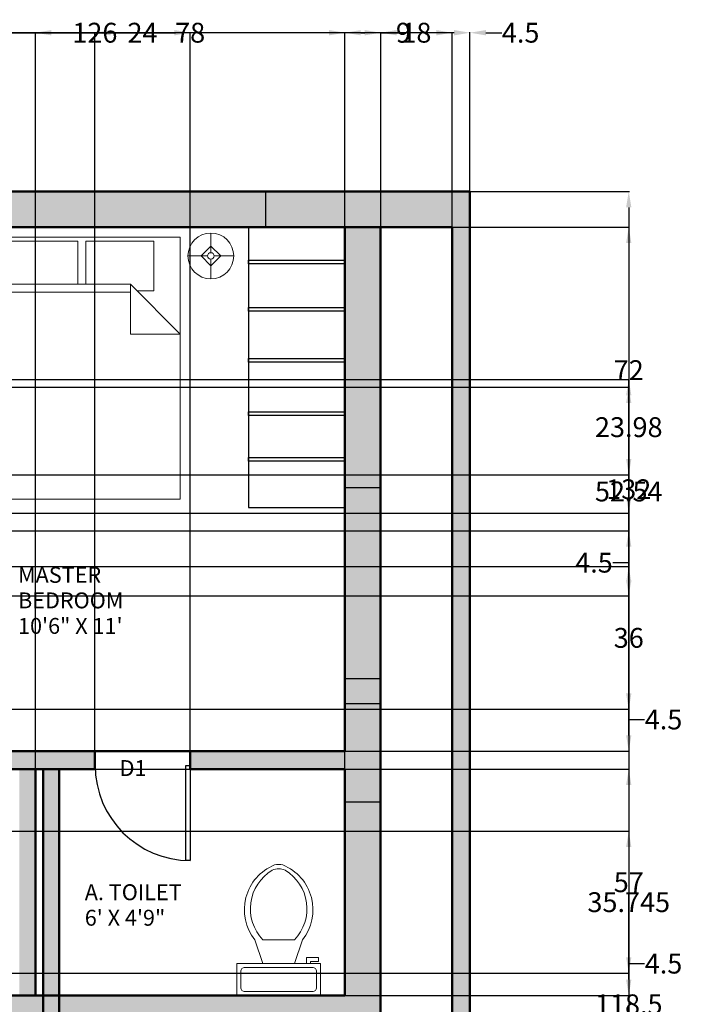
# Model space of a CAD drawing. Units: inches. Extents: x -12 to 887, y 330 to 874.
# Tile 9 of 9: x 720 to 887, y 626 to 874. Entities that reach past the tile are written whole.
import ezdxf

# ---------------------------------------------------------------- set-up
doc = ezdxf.new("R2010")
doc.units = ezdxf.units.IN
doc.header["$MEASUREMENT"] = 0
for name, color, linetype, lineweight in [('A-ANNO-DIMS', 2, 'Continuous', 18), ('A-ANNO-TEXT', 3, 'Continuous', 18), ('A-AREA-IDEN', 7, 'Continuous', 18), ('A-DOOR', 4, 'Continuous', 25), ('A-FLOR-FIXT', 8, 'Continuous', 18), ('A-FLOR-STRS', 3, 'Continuous', 25), ('A-FURN', 9, 'Continuous', 18), ('A-GLAZ', 4, 'Continuous', 25), ('A-WALL', 7, 'Continuous', 50), ('A-WALL-PATT', 5, 'Continuous', 13)]:
    doc.layers.add(name, color=color, linetype=linetype, lineweight=lineweight)
doc.styles.get("Standard").update_dxf_attribs({"font": 'arial.ttf'})
doc.dimstyles.get("Standard").update_dxf_attribs({"dimtxt": 5, "dimasz": 4, "dimexe": 0.18, "dimexo": 0.0625, "dimgap": 0.09, "dimtad": 0, "dimtih": 1, "dimtoh": 1, "dimdec": 1, "dimzin": 0, "dimdsep": 46, "dimlunit": 4, "dimtxsty": 'Standard', "dimcen": 0.09, "dimadec": 0, "dimazin": 0, "dimtfac": 1, "dimtdec": 1, "dimtofl": 0, "dimtmove": 0, "dimatfit": 3, "dimfxl": 1, "dimtolj": 1, "dimtzin": 0, "dimarcsym": 0})

# ---------------------------------------------------------------- blocks, each defined once
blk = doc.blocks.new('*U5')
for p, q in [((0, 0), (0, -6)), ((40, 0), (40, -6))]:
    blk.add_line(p, q)
blk.add_lwpolyline([(0, 0), (0, 40), (1.75, 40), (1.75, 0)], close=True)
blk.add_arc((0, 0), 40, 0, 90)
blk = doc.blocks.new('Bed - Queen')
for p, q in [((0, -80.00003), (0, 0)), ((0, 0), (59.99999, 0)), ((59.99999, 0), (59.99999, -80.00003)), ((7.99999, -1.2), (28.79998, -1.2)), ((7.99999, -14.4), (7.99999, -1.2)), ((28.79998, -1.2), (28.79998, -14.4)), ((31.19999, -1.2), (51.99999, -1.2)), ((31.19999, -14.4), (31.19999, -1.2)), ((51.99999, -1.2), (51.99999, -16.4)), ((0, -14.4), (44.8, -14.4)), ((59.99999, -29.6), (44.8, -14.4)), ((44.8, -14.4), (44.8, -29.6)), ((44.8, -16.8), (0, -16.8)), ((51.99999, -16.4), (46.79936, -16.4)), ((44.8, -29.6), (59.99999, -29.6)), ((59.99999, -80.00003), (0, -80.00003))]:
    blk.add_line(p, q)
blk = doc.blocks.new('Lamp - Table')
for p, q in [((0, 7), (0, 1)), ((-1, 0), (-7, 0)), ((0, 3), (-3, 0)), ((-3, 0), (0, -3)), ((3, 0), (0, 3)), ((0, -3), (3, 0)), ((1, 0), (7, 0)), ((0, -1), (0, -7))]:
    blk.add_line(p, q)
for radius in [7, 1]:
    blk.add_circle((0, 0), radius)
blk = doc.blocks.new('*U12')
for p, q in [((241.3, -152.4), (241.3, -50.8)), ((-254, -215.9), (-203.2, -215.9)), ((-254, -241.3), (-254, -215.9)), ((-177.8, -241.3), (-254, -241.3)), ((-203.2, -215.9), (-203.2, -203.2)), ((-177.8, -203.2), (-177.8, -241.3)), ((-101.6, -203.2), (-152.4, -355.6)), ((101.6, -203.2), (152.4, -355.6)), ((101.6, -355.6), (-101.6, -355.6))]:
    blk.add_line(p, q)
blk.add_lwpolyline([(266.7, -203.2), (266.7, 0), (-266.7, 0), (-266.7, -203.2)], close=True)
for points in [[(-241.3, -50.8), (-241.3, -152.4)], [(215.9, -25.4), (-215.9, -25.4)], [(-215.9, -177.8), (215.9, -177.8)]]:
    blk.add_lwpolyline(points)
for centre, radius, start, end in [((-219.1, -47.6), 22.5, 81.8699, 188.1301), ((219.1, -47.6), 22.5, 351.8699, 98.1301), ((-219.1, -155.6), 22.5, 171.8699, 278.1301), ((219.1, -155.6), 22.5, 261.8699, 8.1301), ((89.4, -548.1), 309.1, 141.46911, 247.97143), ((106.7, -554.2), 287.8, 136.36773, 238.94682), ((-89.4, -548.1), 309.1, 292.02843, 38.53071), ((-106.7, -554.2), 287.8, 301.05301, 43.63209), ((0, -708.1), 101.6, 245.73182, 294.26817), ((0, -736.6), 101.6, 254.86053, 285.13947)]:
    blk.add_arc(centre, radius, start, end)
blk = doc.blocks.new('*D64')
at = {"layer": 'A-ANNO-DIMS', "color": 0, "lineweight": -2, "transparency": 16777216}
for p, q in [((383.99, 685.16), (873.75, 685.16)), ((873.57, 681.16), (873.57, 628.55)), ((873.57, 570.66), (873.57, 623.27)), ((383.99, 566.66), (873.75, 566.66))]:
    blk.add_line(p, q, dxfattribs=at)
at = {"layer": 'A-ANNO-DIMS', "color": 0, "transparency": 16777216}
for points in [[(872.9, 681.16), (874.24, 681.16), (873.57, 685.16)], [(872.9, 570.66), (874.24, 570.66), (873.57, 566.66)]]:
    blk.add_solid(points, dxfattribs=at)
at = {"layer": 'Defpoints', "color": 0, "transparency": 16777216}
for p in [(383.93, 685.16), (873.57, 685.16), (383.93, 566.66)]:
    blk.add_point(p, dxfattribs=at)
at = {"layer": 'A-ANNO-DIMS', "color": 0, "transparency": 16777216, "insert": (873.57, 625.91), "char_height": 5, "attachment_point": 5}
blk.add_mtext('\\A1;118.5', dxfattribs=at)
blk = doc.blocks.new('*D65')
at = {"layer": 'A-ANNO-DIMS', "color": 0, "lineweight": -2, "transparency": 16777216}
for p, q in [((873.57, 693.66), (873.57, 697.66)), ((873.57, 697.66), (877.57, 697.66)), ((383.99, 689.66), (873.75, 689.66)), ((383.99, 685.16), (873.75, 685.16)), ((873.57, 681.16), (873.57, 677.16))]:
    blk.add_line(p, q, dxfattribs=at)
at = {"layer": 'A-ANNO-DIMS', "color": 0, "transparency": 16777216}
for points in [[(872.9, 693.66), (874.24, 693.66), (873.57, 689.66)], [(872.9, 681.16), (874.24, 681.16), (873.57, 685.16)]]:
    blk.add_solid(points, dxfattribs=at)
at = {"layer": 'Defpoints', "color": 0, "transparency": 16777216}
for p in [(383.93, 689.66), (873.57, 689.66), (383.93, 685.16)]:
    blk.add_point(p, dxfattribs=at)
at = {"layer": 'A-ANNO-DIMS', "color": 0, "transparency": 16777216, "insert": (882.33, 697.66), "char_height": 5, "attachment_point": 5}
blk.add_mtext('\\A1;4.5', dxfattribs=at)
blk = doc.blocks.new('*D66')
at = {"layer": 'A-ANNO-DIMS', "color": 0, "lineweight": -2, "transparency": 16777216}
for p, q in [((383.99, 821.66), (873.75, 821.66)), ((873.57, 817.66), (873.57, 758.31)), ((873.57, 693.66), (873.57, 753.02)), ((383.99, 689.66), (873.75, 689.66))]:
    blk.add_line(p, q, dxfattribs=at)
at = {"layer": 'A-ANNO-DIMS', "color": 0, "transparency": 16777216}
for points in [[(872.9, 817.66), (874.24, 817.66), (873.57, 821.66)], [(872.9, 693.66), (874.24, 693.66), (873.57, 689.66)]]:
    blk.add_solid(points, dxfattribs=at)
at = {"layer": 'Defpoints', "color": 0, "transparency": 16777216}
for p in [(383.93, 821.66), (873.57, 821.66), (383.93, 689.66)]:
    blk.add_point(p, dxfattribs=at)
at = {"layer": 'A-ANNO-DIMS', "color": 0, "transparency": 16777216, "insert": (873.57, 755.66), "char_height": 5, "attachment_point": 5}
blk.add_mtext('\\A1;132', dxfattribs=at)
blk = doc.blocks.new('*D83')
at = {"layer": 'A-ANNO-DIMS', "color": 0, "lineweight": -2, "transparency": 16777216}
for p, q in [((460.07, 830.72), (460.07, 870.84)), ((464.07, 870.66), (638.28, 870.66)), ((829.57, 870.66), (655.36, 870.66)), ((833.57, 830.72), (833.57, 870.84))]:
    blk.add_line(p, q, dxfattribs=at)
at = {"layer": 'A-ANNO-DIMS', "color": 0, "transparency": 16777216}
for points in [[(464.07, 871.33), (464.07, 869.99), (460.07, 870.66)], [(829.57, 871.33), (829.57, 869.99), (833.57, 870.66)]]:
    blk.add_solid(points, dxfattribs=at)
at = {"layer": 'Defpoints', "color": 0, "transparency": 16777216}
for p in [(833.57, 870.66), (460.07, 830.66), (833.57, 830.66)]:
    blk.add_point(p, dxfattribs=at)
at = {"layer": 'A-ANNO-DIMS', "color": 0, "transparency": 16777216, "insert": (646.82, 870.66), "char_height": 5, "attachment_point": 5}
blk.add_mtext('\\A1;373.5', dxfattribs=at)
blk = doc.blocks.new('*D91')
at = {"layer": 'A-ANNO-DIMS', "color": 0, "lineweight": -2, "transparency": 16777216}
for p, q in [((676.07, 821.72), (676.07, 870.84)), ((680.07, 870.66), (733.69, 870.66)), ((798.07, 870.66), (744.44, 870.66)), ((802.07, 821.72), (802.07, 870.84))]:
    blk.add_line(p, q, dxfattribs=at)
at = {"layer": 'A-ANNO-DIMS', "color": 0, "transparency": 16777216}
for points in [[(680.07, 871.33), (680.07, 869.99), (676.07, 870.66)], [(798.07, 871.33), (798.07, 869.99), (802.07, 870.66)]]:
    blk.add_solid(points, dxfattribs=at)
at = {"layer": 'Defpoints', "color": 0, "transparency": 16777216}
for p in [(802.07, 870.66), (676.07, 821.66), (802.07, 821.66)]:
    blk.add_point(p, dxfattribs=at)
at = {"layer": 'A-ANNO-DIMS', "color": 0, "transparency": 16777216, "insert": (739.07, 870.66), "char_height": 5, "attachment_point": 5}
blk.add_mtext('\\A1;126', dxfattribs=at)
blk = doc.blocks.new('*D92')
at = {"layer": 'A-ANNO-DIMS', "color": 0, "lineweight": -2, "transparency": 16777216}
for p, q in [((802.07, 821.72), (802.07, 870.84)), ((806.07, 870.66), (807.07, 870.66)), ((811.07, 821.72), (811.07, 870.84)), ((811.07, 870.66), (815.07, 870.66))]:
    blk.add_line(p, q, dxfattribs=at)
at = {"layer": 'A-ANNO-DIMS', "color": 0, "transparency": 16777216}
for points in [[(806.07, 871.33), (806.07, 869.99), (802.07, 870.66)], [(807.07, 871.33), (807.07, 869.99), (811.07, 870.66)]]:
    blk.add_solid(points, dxfattribs=at)
at = {"layer": 'Defpoints', "color": 0, "transparency": 16777216}
for p in [(811.07, 870.66), (802.07, 821.66), (811.07, 821.66)]:
    blk.add_point(p, dxfattribs=at)
at = {"layer": 'A-ANNO-DIMS', "color": 0, "transparency": 16777216, "insert": (816.8, 870.66), "char_height": 5, "attachment_point": 5}
blk.add_mtext('\\A1;9', dxfattribs=at)
blk = doc.blocks.new('*D93')
at = {"layer": 'A-ANNO-DIMS', "color": 0, "lineweight": -2, "transparency": 16777216}
for p, q in [((811.07, 821.72), (811.07, 870.84)), ((815.07, 870.66), (816.63, 870.66)), ((825.07, 870.66), (823.51, 870.66)), ((829.07, 821.72), (829.07, 870.84))]:
    blk.add_line(p, q, dxfattribs=at)
at = {"layer": 'A-ANNO-DIMS', "color": 0, "transparency": 16777216}
for points in [[(815.07, 871.33), (815.07, 869.99), (811.07, 870.66)], [(825.07, 871.33), (825.07, 869.99), (829.07, 870.66)]]:
    blk.add_solid(points, dxfattribs=at)
at = {"layer": 'Defpoints', "color": 0, "transparency": 16777216}
for p in [(829.07, 870.66), (811.07, 821.66), (829.07, 821.66)]:
    blk.add_point(p, dxfattribs=at)
at = {"layer": 'A-ANNO-DIMS', "color": 0, "transparency": 16777216, "insert": (820.07, 870.66), "char_height": 5, "attachment_point": 5}
blk.add_mtext('\\A1;18', dxfattribs=at)
blk = doc.blocks.new('*D94')
at = {"layer": 'A-ANNO-DIMS', "color": 0, "lineweight": -2, "transparency": 16777216}
for p, q in [((825.07, 870.66), (821.07, 870.66)), ((829.07, 821.72), (829.07, 870.84)), ((833.57, 830.72), (833.57, 870.84)), ((837.57, 870.66), (841.57, 870.66))]:
    blk.add_line(p, q, dxfattribs=at)
at = {"layer": 'A-ANNO-DIMS', "color": 0, "transparency": 16777216}
for points in [[(825.07, 871.33), (825.07, 869.99), (829.07, 870.66)], [(837.57, 871.33), (837.57, 869.99), (833.57, 870.66)]]:
    blk.add_solid(points, dxfattribs=at)
at = {"layer": 'Defpoints', "color": 0, "transparency": 16777216}
for p in [(833.57, 870.66), (833.57, 830.66), (829.07, 821.66)]:
    blk.add_point(p, dxfattribs=at)
at = {"layer": 'A-ANNO-DIMS', "color": 0, "transparency": 16777216, "insert": (846.33, 870.66), "char_height": 5, "attachment_point": 5}
blk.add_mtext('\\A1;4.5', dxfattribs=at)
blk = doc.blocks.new('*D98')
at = {"layer": 'A-ANNO-DIMS', "color": 0, "lineweight": -2, "transparency": 16777216}
for p, q in [((460.13, 830.66), (873.75, 830.66)), ((873.57, 826.66), (873.57, 604.54)), ((873.57, 377.16), (873.57, 599.28)), ((460.13, 373.16), (873.75, 373.16))]:
    blk.add_line(p, q, dxfattribs=at)
at = {"layer": 'A-ANNO-DIMS', "color": 0, "transparency": 16777216}
for points in [[(872.9, 826.66), (874.24, 826.66), (873.57, 830.66)], [(872.9, 377.16), (874.24, 377.16), (873.57, 373.16)]]:
    blk.add_solid(points, dxfattribs=at)
at = {"layer": 'Defpoints', "color": 0, "transparency": 16777216}
for p in [(460.07, 830.66), (873.57, 830.66), (460.07, 373.16)]:
    blk.add_point(p, dxfattribs=at)
at = {"layer": 'A-ANNO-DIMS', "color": 0, "transparency": 16777216, "insert": (873.57, 601.91), "char_height": 5, "attachment_point": 5}
blk.add_mtext('\\A1;457.5', dxfattribs=at)
blk = doc.blocks.new('*D109')
at = {"layer": 'A-ANNO-DIMS', "color": 0, "lineweight": -2, "transparency": 16777216}
for p, q in [((873.57, 632.16), (873.57, 636.16)), ((873.57, 636.16), (877.57, 636.16)), ((802.13, 628.16), (873.75, 628.16)), ((802.13, 623.66), (873.75, 623.66)), ((873.57, 619.66), (873.57, 615.66))]:
    blk.add_line(p, q, dxfattribs=at)
at = {"layer": 'A-ANNO-DIMS', "color": 0, "transparency": 16777216}
for points in [[(872.9, 632.16), (874.24, 632.16), (873.57, 628.16)], [(872.9, 619.66), (874.24, 619.66), (873.57, 623.66)]]:
    blk.add_solid(points, dxfattribs=at)
at = {"layer": 'Defpoints', "color": 0, "transparency": 16777216}
for p in [(802.07, 628.16), (873.57, 628.16), (802.07, 623.66)]:
    blk.add_point(p, dxfattribs=at)
at = {"layer": 'A-ANNO-DIMS', "color": 0, "transparency": 16777216, "insert": (882.33, 636.16), "char_height": 5, "attachment_point": 5}
blk.add_mtext('\\A1;4.5', dxfattribs=at)
blk = doc.blocks.new('*D110')
at = {"layer": 'A-ANNO-DIMS', "color": 0, "lineweight": -2, "transparency": 16777216}
for p, q in [((802.13, 685.16), (873.75, 685.16)), ((873.57, 681.16), (873.57, 659.29)), ((873.57, 632.16), (873.57, 654.03)), ((802.13, 628.16), (873.75, 628.16))]:
    blk.add_line(p, q, dxfattribs=at)
at = {"layer": 'A-ANNO-DIMS', "color": 0, "transparency": 16777216}
for points in [[(872.9, 681.16), (874.24, 681.16), (873.57, 685.16)], [(872.9, 632.16), (874.24, 632.16), (873.57, 628.16)]]:
    blk.add_solid(points, dxfattribs=at)
at = {"layer": 'Defpoints', "color": 0, "transparency": 16777216}
for p in [(802.07, 685.16), (873.57, 685.16), (802.07, 628.16)]:
    blk.add_point(p, dxfattribs=at)
at = {"layer": 'A-ANNO-DIMS', "color": 0, "transparency": 16777216, "insert": (873.57, 656.66), "char_height": 5, "attachment_point": 5}
blk.add_mtext('\\A1;57', dxfattribs=at)
blk = doc.blocks.new('*D111')
at = {"layer": 'A-ANNO-DIMS', "color": 0, "lineweight": -2, "transparency": 16777216}
for p, q in [((873.57, 693.66), (873.57, 697.66)), ((873.57, 697.66), (877.57, 697.66)), ((802.13, 689.66), (873.75, 689.66)), ((802.13, 685.16), (873.75, 685.16)), ((873.57, 681.16), (873.57, 677.16))]:
    blk.add_line(p, q, dxfattribs=at)
at = {"layer": 'A-ANNO-DIMS', "color": 0, "transparency": 16777216}
for points in [[(872.9, 693.66), (874.24, 693.66), (873.57, 689.66)], [(872.9, 681.16), (874.24, 681.16), (873.57, 685.16)]]:
    blk.add_solid(points, dxfattribs=at)
at = {"layer": 'Defpoints', "color": 0, "transparency": 16777216}
for p in [(802.07, 689.66), (873.57, 689.66), (802.07, 685.16)]:
    blk.add_point(p, dxfattribs=at)
at = {"layer": 'A-ANNO-DIMS', "color": 0, "transparency": 16777216, "insert": (882.33, 697.66), "char_height": 5, "attachment_point": 5}
blk.add_mtext('\\A1;4.5', dxfattribs=at)
blk = doc.blocks.new('*D114')
at = {"layer": 'A-ANNO-DIMS', "color": 0, "lineweight": -2, "transparency": 16777216}
for p, q in [((724.07, 628.22), (724.07, 870.84)), ((728.07, 870.66), (759.41, 870.66)), ((798.07, 870.66), (766.72, 870.66)), ((802.07, 628.22), (802.07, 870.84))]:
    blk.add_line(p, q, dxfattribs=at)
at = {"layer": 'A-ANNO-DIMS', "color": 0, "transparency": 16777216}
for points in [[(728.07, 871.33), (728.07, 869.99), (724.07, 870.66)], [(798.07, 871.33), (798.07, 869.99), (802.07, 870.66)]]:
    blk.add_solid(points, dxfattribs=at)
at = {"layer": 'Defpoints', "color": 0, "transparency": 16777216}
for p in [(802.07, 870.66), (724.07, 628.16), (802.07, 628.16)]:
    blk.add_point(p, dxfattribs=at)
at = {"layer": 'A-ANNO-DIMS', "color": 0, "transparency": 16777216, "insert": (763.07, 870.66), "char_height": 5, "attachment_point": 5}
blk.add_mtext('\\A1;78', dxfattribs=at)
blk = doc.blocks.new('*D116')
at = {"layer": 'A-ANNO-DIMS', "color": 0, "lineweight": -2, "transparency": 16777216}
for p, q in [((873.57, 753.66), (873.57, 757.66)), ((621.63, 749.66), (873.75, 749.66)), ((617.13, 745.16), (873.75, 745.16)), ((873.57, 741.16), (873.57, 737.16)), ((873.57, 737.16), (869.57, 737.16))]:
    blk.add_line(p, q, dxfattribs=at)
at = {"layer": 'A-ANNO-DIMS', "color": 0, "transparency": 16777216}
for points in [[(872.9, 753.66), (874.24, 753.66), (873.57, 749.66)], [(872.9, 741.16), (874.24, 741.16), (873.57, 745.16)]]:
    blk.add_solid(points, dxfattribs=at)
at = {"layer": 'Defpoints', "color": 0, "transparency": 16777216}
for p in [(621.57, 749.66), (617.07, 745.16), (873.57, 745.16)]:
    blk.add_point(p, dxfattribs=at)
at = {"layer": 'A-ANNO-DIMS', "color": 0, "transparency": 16777216, "insert": (864.81, 737.16), "char_height": 5, "attachment_point": 5}
blk.add_mtext('\\A1;4.5', dxfattribs=at)
blk = doc.blocks.new('*D117')
at = {"layer": 'A-ANNO-DIMS', "color": 0, "lineweight": -2, "transparency": 16777216}
for p, q in [((621.63, 821.66), (873.75, 821.66)), ((873.57, 817.66), (873.57, 788.26)), ((873.57, 753.66), (873.57, 783.06)), ((621.63, 749.66), (873.75, 749.66))]:
    blk.add_line(p, q, dxfattribs=at)
at = {"layer": 'A-ANNO-DIMS', "color": 0, "transparency": 16777216}
for points in [[(872.9, 817.66), (874.24, 817.66), (873.57, 821.66)], [(872.9, 753.66), (874.24, 753.66), (873.57, 749.66)]]:
    blk.add_solid(points, dxfattribs=at)
at = {"layer": 'Defpoints', "color": 0, "transparency": 16777216}
for p in [(621.57, 821.66), (873.57, 821.66), (621.57, 749.66)]:
    blk.add_point(p, dxfattribs=at)
at = {"layer": 'A-ANNO-DIMS', "color": 0, "transparency": 16777216, "insert": (873.57, 785.66), "char_height": 5, "attachment_point": 5}
blk.add_mtext('\\A1;72', dxfattribs=at)
blk = doc.blocks.new('*D122')
at = {"layer": 'A-ANNO-DIMS', "color": 0, "lineweight": -2, "transparency": 16777216}
for p, q in [((671.63, 736.22), (873.75, 736.22)), ((873.57, 732.22), (873.57, 720.87)), ((873.57, 704.22), (873.57, 715.58)), ((671.63, 700.22), (873.75, 700.22))]:
    blk.add_line(p, q, dxfattribs=at)
at = {"layer": 'A-ANNO-DIMS', "color": 0, "transparency": 16777216}
for points in [[(872.9, 732.22), (874.24, 732.22), (873.57, 736.22)], [(872.9, 704.22), (874.24, 704.22), (873.57, 700.22)]]:
    blk.add_solid(points, dxfattribs=at)
at = {"layer": 'Defpoints', "color": 0, "transparency": 16777216}
for p in [(671.57, 736.22), (671.57, 700.22), (873.57, 700.22)]:
    blk.add_point(p, dxfattribs=at)
at = {"layer": 'A-ANNO-DIMS', "color": 0, "transparency": 16777216, "insert": (873.57, 718.22), "char_height": 5, "attachment_point": 5}
blk.add_mtext('\\A1;36', dxfattribs=at)
blk = doc.blocks.new('*D123')
at = {"layer": 'A-ANNO-DIMS', "color": 0, "lineweight": -2, "transparency": 16777216}
for p, q in [((617.13, 783.29), (873.75, 783.29)), ((873.57, 779.29), (873.57, 773.94)), ((873.57, 763.31), (873.57, 768.65)), ((617.13, 759.31), (873.75, 759.31))]:
    blk.add_line(p, q, dxfattribs=at)
at = {"layer": 'A-ANNO-DIMS', "color": 0, "transparency": 16777216}
for points in [[(872.9, 779.29), (874.24, 779.29), (873.57, 783.29)], [(872.9, 763.31), (874.24, 763.31), (873.57, 759.31)]]:
    blk.add_solid(points, dxfattribs=at)
at = {"layer": 'Defpoints', "color": 0, "transparency": 16777216}
for p in [(617.07, 783.29), (617.07, 759.31), (873.57, 759.31)]:
    blk.add_point(p, dxfattribs=at)
at = {"layer": 'A-ANNO-DIMS', "color": 0, "transparency": 16777216, "insert": (873.57, 771.3), "char_height": 5, "attachment_point": 5}
blk.add_mtext('\\A1;23.98', dxfattribs=at)
blk = doc.blocks.new('*D126')
at = {"layer": 'A-ANNO-DIMS', "color": 0, "lineweight": -2, "transparency": 16777216}
for p, q in [((739.07, 685.22), (739.07, 870.84)), ((743.07, 870.66), (747.36, 870.66)), ((759.07, 870.66), (754.77, 870.66)), ((763.07, 685.22), (763.07, 870.84))]:
    blk.add_line(p, q, dxfattribs=at)
at = {"layer": 'A-ANNO-DIMS', "color": 0, "transparency": 16777216}
for points in [[(743.07, 871.33), (743.07, 869.99), (739.07, 870.66)], [(759.07, 871.33), (759.07, 869.99), (763.07, 870.66)]]:
    blk.add_solid(points, dxfattribs=at)
at = {"layer": 'Defpoints', "color": 0, "transparency": 16777216}
for p in [(763.07, 870.66), (739.07, 685.16), (763.07, 685.16)]:
    blk.add_point(p, dxfattribs=at)
at = {"layer": 'A-ANNO-DIMS', "color": 0, "transparency": 16777216, "insert": (751.07, 870.66), "char_height": 5, "attachment_point": 5}
blk.add_mtext('\\A1;24', dxfattribs=at)
blk = doc.blocks.new('*D127')
at = {"layer": 'A-ANNO-DIMS', "color": 0, "lineweight": -2, "transparency": 16777216}
for p, q in [((671.63, 669.51), (873.75, 669.51)), ((873.57, 665.51), (873.57, 654.28)), ((873.57, 637.77), (873.57, 648.99)), ((671.63, 633.77), (873.75, 633.77))]:
    blk.add_line(p, q, dxfattribs=at)
at = {"layer": 'A-ANNO-DIMS', "color": 0, "transparency": 16777216}
for points in [[(872.9, 665.51), (874.24, 665.51), (873.57, 669.51)], [(872.9, 637.77), (874.24, 637.77), (873.57, 633.77)]]:
    blk.add_solid(points, dxfattribs=at)
at = {"layer": 'Defpoints', "color": 0, "transparency": 16777216}
for p in [(671.57, 669.51), (671.57, 633.77), (873.57, 633.77)]:
    blk.add_point(p, dxfattribs=at)
at = {"layer": 'A-ANNO-DIMS', "color": 0, "transparency": 16777216, "insert": (873.57, 651.64), "char_height": 5, "attachment_point": 5}
blk.add_mtext('\\A1;35.745', dxfattribs=at)
blk = doc.blocks.new('*D128')
at = {"layer": 'A-ANNO-DIMS', "color": 0, "lineweight": -2, "transparency": 16777216}
for p, q in [((488.63, 781.36), (873.75, 781.36)), ((873.57, 777.36), (873.57, 757.74)), ((873.57, 732.83), (873.57, 752.45)), ((488.63, 728.83), (873.75, 728.83))]:
    blk.add_line(p, q, dxfattribs=at)
at = {"layer": 'A-ANNO-DIMS', "color": 0, "transparency": 16777216}
for points in [[(872.9, 777.36), (874.24, 777.36), (873.57, 781.36)], [(872.9, 732.83), (874.24, 732.83), (873.57, 728.83)]]:
    blk.add_solid(points, dxfattribs=at)
at = {"layer": 'Defpoints', "color": 0, "transparency": 16777216}
for p in [(488.57, 781.36), (488.57, 728.83), (873.57, 728.83)]:
    blk.add_point(p, dxfattribs=at)
at = {"layer": 'A-ANNO-DIMS', "color": 0, "transparency": 16777216, "insert": (873.57, 755.1), "char_height": 5, "attachment_point": 5}
blk.add_mtext('\\A1;52.54', dxfattribs=at)

msp = doc.modelspace()

# ---------------------------------------------------------------- hatches: boundary and pattern name
at = {"layer": 'A-WALL-PATT'}
h = msp.add_hatch(color=256, dxfattribs=at)
h.dxf.hatch_style = 1
h.paths.add_polyline_path([(94.575, 830.6611), (67.3199, 830.6611), (67.3199, 821.6611), (70.4263, 821.6611), (79.4263, 821.6611), (94.575, 821.6611)])
h.paths.add_polyline_path([(288.8031, 830.6611), (257.9263, 830.6611), (253.4263, 830.6611), (253.4263, 821.6611), (288.8031, 821.6611)])
h.paths.add_polyline_path([(74.9263, 696.9265), (70.4263, 696.9265), (70.4263, 678.4656), (74.9263, 678.4656)])
h.paths.add_polyline_path([(74.9263, 584.8756), (70.4263, 584.8756), (70.4263, 562.1611), (74.9263, 562.1611)])
h.paths.add_polyline_path([(135.5357, 566.6611), (122.6994, 566.6611), (122.6994, 562.1611), (135.5357, 562.1611)])
h.paths.add_polyline_path([(257.9263, 579.1607), (253.4263, 579.1607), (253.4263, 562.1611), (257.9263, 562.1611)])
h.paths.add_polyline_path([(272.0195, 454.1611), (254.2006, 454.1611), (254.2006, 450.1611), (272.0195, 450.1611)])
h.paths.add_polyline_path([(392.9263, 454.1611), (374.959, 454.1611), (374.959, 450.1611), (383.9263, 450.1611), (392.9263, 450.1611)])
h.paths.add_polyline_path([(493.0683, 466.4171), (488.5683, 466.4171), (488.5683, 450.1611), (493.0683, 450.1611)])
h.paths.add_polyline_path([(568.6302, 454.1611), (555.938, 454.1611), (555.938, 450.1611), (568.6302, 450.1611)])
h.paths.add_polyline_path([(493.0683, 594.9471), (488.5683, 594.9471), (488.5683, 569.5862), (493.0683, 569.5862)])
h.paths.add_polyline_path([(690.1615, 454.1611), (672.3426, 454.1611), (672.3426, 450.1611), (690.1615, 450.1611)])
h.paths.add_polyline_path([(811.0683, 454.1611), (793.101, 454.1611), (793.101, 450.1611), (802.0683, 450.1611), (811.0683, 450.1611)])
h.paths.add_polyline_path([(811.0683, 578.3606), (802.0683, 578.3606), (802.0683, 566.6611), (802.0683, 553.5254), (811.0683, 553.5254)])
h.paths.add_polyline_path([(811.0683, 701.6611), (802.0683, 701.6611), (802.0683, 689.9616), (802.0683, 676.8259), (811.0683, 676.8259)])
h.paths.add_polyline_path([(811.0683, 830.6611), (782.165, 830.6611), (782.165, 821.6611), (802.0683, 821.6611), (811.0683, 821.6611)])
h.paths.add_polyline_path([(706.9451, 830.6611), (671.5683, 830.6611), (671.5683, 821.6611), (706.9451, 821.6611)])
h.paths.add_polyline_path([(512.717, 830.6611), (485.4619, 830.6611), (485.4619, 821.6611), (488.5683, 821.6611), (512.717, 821.6611)])
h.paths.add_polyline_path([(392.9263, 697.8668), (383.9263, 697.8668), (383.9263, 689.6611), (383.9263, 676.5034), (392.9263, 676.5034)])
h.paths.add_polyline_path([(392.9263, 830.6611), (364.023, 830.6611), (364.023, 821.7357), (392.9263, 821.7357)])
h.paths.add_polyline_path([(392.9263, 619.0434), (383.9263, 619.0434), (383.9263, 588.7499), (392.9263, 588.7499)])
h.paths.add_polyline_path([(392.9263, 578.3606), (383.9263, 578.3606), (383.9263, 566.6611), (383.9263, 553.5254), (392.9263, 553.5254)])
h.paths.add_polyline_path([(257.9263, 699.8547), (253.4263, 699.8547), (253.4263, 697.1611), (253.4263, 677.338), (257.9263, 677.338)])
h.paths.add_polyline_path([(493.0683, 714.3785), (488.5683, 714.3785), (488.5683, 689.6611), (493.0683, 689.6611)])
h.paths.add_polyline_path([(74.9263, 491.4191), (70.4263, 491.4191), (70.4263, 480.7097), (74.9263, 480.7097)])
h = msp.add_hatch(color=256, dxfattribs=at)
h.dxf.hatch_style = 1
h.paths.add_polyline_path([(671.5683, 830.6611), (512.717, 830.6611), (512.717, 821.6611), (617.0825, 821.6611), (617.0825, 797.5825), (617.0787, 783.3094), (621.5683, 783.3094), (621.5683, 821.6611), (671.5683, 821.6611)], flags=17)
h.paths.add_polyline_path([(833.5683, 830.6611), (811.0683, 830.6611), (811.0683, 821.6611), (829.0683, 821.6611), (829.0683, 701.6611), (829.0683, 382.1611), (811.0683, 382.1611), (811.0683, 450.1611), (802.0683, 450.1611), (802.0683, 382.1611), (671.5683, 382.1611), (464.5683, 382.1611), (464.5683, 821.6611), (460.0683, 821.6611), (460.0683, 373.1611), (671.5683, 373.1611), (833.5683, 373.1611)])
h.paths.add_polyline_path([(493.0683, 728.8273), (488.5683, 728.8273), (488.5683, 714.3785), (493.0683, 714.3785)], flags=17)
h.paths.add_polyline_path([(493.0683, 821.6611), (488.5683, 821.6611), (488.5683, 781.3634), (493.0683, 781.3634)], flags=17)
h = msp.add_hatch(color=256, dxfattribs=at)
h.dxf.hatch_style = 1
h.paths.add_polyline_path([(485.4619, 830.6611), (460.0683, 830.6611), (460.0683, 373.1611), (833.5683, 373.1611), (833.5683, 830.6611), (811.0683, 830.6611), (811.0683, 821.6611), (829.0683, 821.6611), (829.0683, 701.6611), (829.0683, 382.1611), (811.0683, 382.1611), (811.0683, 450.1611), (802.0683, 450.1611), (802.0683, 382.1611), (671.5683, 382.1611), (464.5683, 382.1611), (464.5683, 821.6611), (485.4619, 821.6611)])
h = msp.add_hatch(color=256, dxfattribs=at)
h.dxf.hatch_style = 1
h.paths.add_polyline_path([(671.5683, 749.6611), (621.5683, 749.6611), (621.5683, 759.3094), (620.6653, 759.3094), (617.0683, 759.3094), (617.0683, 745.1611), (671.5683, 745.1611)])
h.paths.add_polyline_path([(676.0683, 821.6611), (671.5683, 821.6611), (671.5683, 736.2424), (676.0683, 736.2424)])
h.paths.add_polyline_path([(782.165, 830.6611), (706.9451, 830.6611), (706.9451, 821.6611), (782.165, 821.6611)])
h.paths.add_polyline_path([(811.0683, 553.5254), (802.0683, 553.5254), (802.0683, 507.4529), (802.0683, 454.1611), (811.0683, 454.1611)])
h.paths.add_polyline_path([(793.101, 454.1611), (690.1615, 454.1611), (690.1615, 450.1611), (793.101, 450.1611)])
h.paths.add_polyline_path([(672.3426, 454.1611), (656.7304, 454.1611), (656.7304, 450.1611), (672.3426, 450.1611)])
h.paths.add_polyline_path([(582.6585, 454.1611), (568.6302, 454.1611), (568.6302, 450.1611), (582.6585, 450.1611)])
h.paths.add_polyline_path([(555.938, 454.1611), (554.2565, 454.1611), (554.2565, 452.8628), (554.2565, 450.1611), (555.938, 450.1611)])
h.paths.add_polyline_path([(518.2335, 452.8628), (518.2335, 454.1611), (493.0683, 454.1611), (493.0683, 450.1611), (518.2335, 450.1611)])
h.paths.add_polyline_path([(493.0683, 450.1611), (488.5683, 450.1611), (488.5683, 382.1611), (493.0683, 382.1611)])
h.paths.add_polyline_path([(493.0683, 492.3446), (488.5683, 492.3446), (488.5683, 466.4171), (493.0683, 466.4171)])
h.paths.add_polyline_path([(493.0683, 569.5862), (488.5683, 569.5862), (488.5683, 557.2595), (493.0683, 557.2595)])
h.paths.add_polyline_path([(493.0683, 689.6611), (488.5683, 689.6611), (488.5683, 594.9471), (493.0683, 594.9471)])
h.paths.add_polyline_path([(676.0683, 700.2227), (671.5683, 700.2227), (671.5683, 669.5589), (676.0683, 669.5589)])
h.paths.add_polyline_path([(739.0683, 689.6611), (676.0683, 689.6611), (676.0683, 685.1611), (739.0683, 685.1611)])
h.paths.add_polyline_path([(802.0683, 689.6611), (763.0683, 689.6611), (763.0683, 686.0698), (763.0683, 685.1611), (802.0683, 685.1611)])
h.paths.add_polyline_path([(811.0683, 821.6611), (802.0683, 821.6611), (802.0683, 756.0738), (811.0683, 756.0738)])
h.paths.add_polyline_path([(811.0683, 707.8935), (802.0683, 707.8935), (802.0683, 701.6611), (811.0683, 701.6611)])
h.paths.add_polyline_path([(811.0683, 676.8259), (802.0683, 676.8259), (802.0683, 628.1611), (730.0683, 628.1611), (730.0683, 623.6611), (802.0683, 623.6611), (802.0683, 578.3606), (811.0683, 578.3606)])
h.paths.add_polyline_path([(730.0683, 685.1611), (726.0683, 685.1611), (726.0683, 628.1611), (730.0683, 628.1611)])
h.paths.add_polyline_path([(724.0683, 685.1611), (720.0683, 685.1611), (720.0683, 628.1611), (724.0683, 628.1611)])
h.paths.add_polyline_path([(726.0683, 628.1611), (676.0683, 628.1611), (676.0683, 633.7662), (674.2492, 633.7662), (671.5683, 633.7662), (671.5683, 623.6611), (726.0683, 623.6611)])
h.paths.add_polyline_path([(730.0683, 628.1611), (726.0683, 628.1611), (726.0683, 623.6611), (730.0683, 623.6611)])
h.paths.add_polyline_path([(730.0683, 623.6611), (726.0683, 623.6611), (726.0683, 595.3822), (729.6731, 595.3822, -0.00411226), (730.0683, 595.379)])
h.paths.add_polyline_path([(802.0683, 564.6611), (730.0683, 564.6611), (730.0683, 571.3507), (729.6731, 571.3507), (726.0683, 571.3507), (726.0683, 564.6611), (718.522, 564.6611), (718.522, 560.1611), (802.0683, 560.1611)])
h.paths.add_polyline_path([(676.0683, 580.4772), (671.5683, 580.4772), (671.5683, 560.1611), (676.0683, 560.1611)])
h.paths.add_polyline_path([(682.5176, 564.6611), (676.0683, 564.6611), (676.0683, 560.1611), (682.5176, 560.1611)])
h.paths.add_polyline_path([(676.0683, 560.1611), (671.5683, 560.1611), (671.5683, 454.1611), (672.3426, 454.1611), (676.0683, 454.1611)])
h = msp.add_hatch(color=256, dxfattribs=at)
h.dxf.hatch_style = 1
h.paths.add_polyline_path([(74.9263, 749.8953), (70.4263, 749.8953), (70.4263, 709.2627), (74.9263, 709.2627)])
h.paths.add_polyline_path([(74.9263, 671.2153), (70.4263, 671.2153), (70.4263, 599.271), (74.9263, 599.271)])
h.paths.add_polyline_path([(229.0035, 566.6611), (142.5107, 566.6611), (142.5107, 562.1611), (229.0035, 562.1611)])
h.paths.add_polyline_path([(392.9263, 742.7561), (383.9263, 742.7561), (383.9263, 706.6608), (392.9263, 706.6608)])
h.paths.add_polyline_path([(656.7304, 454.1611), (582.6585, 454.1611), (582.6585, 450.1611), (656.7304, 450.1611)])
h.paths.add_polyline_path([(493.0683, 557.2595), (488.5683, 557.2595), (488.5683, 492.3446), (493.0683, 492.3446)])
h.paths.add_polyline_path([(493.0683, 781.3634), (488.5683, 781.3634), (488.5683, 728.8273), (493.0683, 728.8273)])
h.paths.add_polyline_path([(811.0683, 756.0738), (802.0683, 756.0738), (802.0683, 707.8935), (811.0683, 707.8935)])

# ---------------------------------------------------------------- linework, layer by layer
at = {"layer": 'A-FLOR-STRS'}
for points in [[(802.0683, 821.6611), (777.8096, 821.6611), (777.8096, 751.0224), (802.0683, 751.0224)], [(777.8096, 813.3906), (802.0683, 813.3906), (802.0683, 812.4725), (777.8096, 812.4725)], [(777.8096, 801.477), (802.0683, 801.477), (802.0683, 800.5589), (777.8096, 800.5589)], [(777.8096, 788.6179), (802.0683, 788.6179), (802.0683, 787.6997), (777.8096, 787.6997)], [(777.8096, 775.1314), (802.0683, 775.1314), (802.0683, 774.2133), (777.8096, 774.2133)], [(777.8096, 763.6836), (802.0683, 763.6836), (802.0683, 762.7655), (777.8096, 762.7655)]]:
    msp.add_lwpolyline(points, close=True, dxfattribs=at)
at = {"layer": 'A-GLAZ'}
for points in [[(782.165, 821.7357), (782.165, 830.6611), (811.0683, 830.6611), (811.0683, 821.7357)], [(802.0683, 689.9616), (802.0683, 701.6611), (811.0683, 701.6611), (811.0683, 676.8259), (802.0683, 676.8259), (802.0683, 689.9616)]]:
    msp.add_lwpolyline(points, dxfattribs=at)
msp.add_lwpolyline([(802.0683, 756.0738), (811.0683, 756.0738), (811.0683, 707.8935), (802.0683, 707.8935)], close=True, dxfattribs=at)
at = {"layer": 'A-WALL'}
for p, q in [((676.0683, 830.6611), (833.5683, 830.6611)), ((833.5683, 830.6611), (833.5683, 373.1611)), ((676.0683, 821.6611), (811.0683, 821.6611)), ((802.0683, 821.6611), (802.0683, 701.6611)), ((811.0683, 821.6611), (811.0683, 382.1611)), ((811.0683, 821.6611), (829.0683, 821.6611)), ((829.0683, 821.6611), (829.0683, 701.6611)), ((802.0683, 701.6611), (802.0683, 689.6611)), ((829.0683, 701.6611), (829.0683, 382.1611)), ((676.0683, 689.6611), (802.0683, 689.6611)), ((739.0683, 689.6611), (739.0683, 685.1611)), ((763.0683, 685.1611), (763.0683, 689.6611)), ((676.0683, 685.1611), (739.0683, 685.1611)), ((724.0683, 685.1611), (724.0683, 628.1611)), ((726.0683, 685.1611), (726.0683, 564.6611)), ((730.0683, 685.1611), (730.0683, 595.3507)), ((763.0683, 685.1611), (802.0683, 685.1611)), ((802.0683, 685.1611), (802.0683, 628.1611)), ((676.0683, 628.1611), (802.0683, 628.1611))]:
    msp.add_line(p, q, dxfattribs=at)

# ---------------------------------------------------------------- block references
at = {"layer": 'A-DOOR', "xscale": 0.5985408836976128, "yscale": 0.5985408836976128, "zscale": 0.5985408836976128, "rotation": 180}
msp.add_blockref('*U5', (763.0683, 686.0698), dxfattribs=at)
at = {"layer": 'A-FLOR-FIXT', "xscale": 0.0393700787401575, "yscale": 0.0393700787401575, "zscale": 0.0393700787401575, "rotation": 180}
msp.add_blockref('*U12', (785.3736, 628.1611), dxfattribs=at)
at = {"layer": 'A-FURN', "xscale": 0.8252380322911079, "yscale": 0.8252380322911079, "zscale": 0.8252380322911079}
for name, p in [('Bed - Queen', (711.048, 819.1735)), ('Lamp - Table', (768.2867, 814.4212))]:
    msp.add_blockref(name, p, dxfattribs=at)

# ---------------------------------------------------------------- texts
at = {"layer": 'A-ANNO-TEXT'}
msp.add_text('D1', height=4, dxfattribs=at).set_placement((745.298, 683.4149))
at = {"layer": 'A-AREA-IDEN'}
for s, p in [('MASTER ', (719.7047, 732.0862)), ('BEDROOM', (719.7047, 725.6605)), ('10\'6" X 11\'', (719.7047, 719.2349)), ('A. TOILET', (736.5189, 652.1391)), ('6\' X 4\'9"', (736.5189, 645.7134))]:
    msp.add_text(s, height=4, dxfattribs=at).set_placement(p)

# ---------------------------------------------------------------- dimensions: what is measured, and where the dimension line sits
at = {"layer": 'A-ANNO-DIMS'}
for base, p1, p2, override, picture, middle in [((833.5683, 870.6611), (460.0683, 830.6611), (833.5683, 830.6611), {"dimdec": 1, "dimlfac": 1, "dimrnd": 0, "dimzin": 0, "dimdsep": 46, "dimlunit": 2}, '*D83', (646.8183, 870.6611)), ((802.0683, 870.6611), (676.0683, 821.6611), (802.0683, 821.6611), {"dimdec": 0, "dimlfac": 1, "dimrnd": 0, "dimzin": 0, "dimdsep": 46, "dimlunit": 2}, '*D91', (739.0683, 870.6611)), ((802.0683, 870.6611), (724.0683, 628.1611), (802.0683, 628.1611), {"dimdec": 0, "dimlfac": 1, "dimrnd": 0, "dimzin": 0, "dimdsep": 46, "dimlunit": 2}, '*D114', (763.0683, 870.6611)), ((763.0683, 870.6611), (739.0683, 685.1611), (763.0683, 685.1611), {"dimdec": 0, "dimlfac": 1, "dimrnd": 0, "dimzin": 0, "dimdsep": 46, "dimlunit": 2}, '*D126', (751.0683, 870.6611)), ((811.0683, 870.6611), (802.0683, 821.6611), (811.0683, 821.6611), {"dimdec": 0, "dimlfac": 1, "dimrnd": 0, "dimzin": 0, "dimdsep": 46, "dimlunit": 2}, '*D92', (816.8023, 870.6611)), ((829.0683, 870.6611), (811.0683, 821.6611), (829.0683, 821.6611), {"dimdec": 0, "dimlfac": 1, "dimrnd": 0, "dimzin": 0, "dimdsep": 46, "dimlunit": 2}, '*D93', (820.0683, 870.6611)), ((833.5683, 870.6611), (829.0683, 821.6611), (833.5683, 830.6611), {"dimdec": 1, "dimlfac": 1, "dimrnd": 0, "dimzin": 0, "dimdsep": 46, "dimlunit": 2}, '*D94', (846.3292, 870.6611))]:
    dim = msp.add_linear_dim(base=base, p1=p1, p2=p2, dimstyle='Standard', override=override, dxfattribs=at)
    dim.commit()
    dim.dimension.update_dxf_attribs({"geometry": picture, "text_midpoint": middle})
for base, p1, p2, override, picture, middle in [((873.5683, 830.6611), (460.0683, 373.1611), (460.0683, 830.6611), {"dimdec": 1, "dimlfac": 1, "dimrnd": 0, "dimzin": 0, "dimdsep": 46, "dimlunit": 2}, '*D98', (873.5683, 601.9111)), ((873.5683, 821.6611), (383.9263, 689.6611), (383.9263, 821.6611), {"dimdec": 0, "dimlfac": 1, "dimrnd": 0, "dimzin": 0, "dimdsep": 46, "dimlunit": 2}, '*D66', (873.5683, 755.6611)), ((873.5683, 821.6611), (621.5683, 749.6611), (621.5683, 821.6611), {"dimdec": 0, "dimlfac": 1, "dimrnd": 0, "dimzin": 0, "dimdsep": 46, "dimlunit": 2}, '*D117', (873.5683, 785.6611)), ((873.5683, 728.8273), (488.5683, 781.3634), (488.5683, 728.8273), {"dimdec": 2, "dimlfac": 1, "dimrnd": 0, "dimzin": 0, "dimdsep": 46, "dimlunit": 2}, '*D128', (873.5683, 755.0953)), ((873.5683, 759.3094), (617.0683, 783.289), (617.0683, 759.3094), {"dimdec": 2, "dimlfac": 1, "dimrnd": 0, "dimzin": 0, "dimdsep": 46, "dimlunit": 2}, '*D123', (873.5683, 771.2992)), ((873.5683, 745.1611), (621.5683, 749.6611), (617.0683, 745.1611), {"dimdec": 1, "dimlfac": 1, "dimrnd": 0, "dimzin": 0, "dimdsep": 46, "dimlunit": 2}, '*D116', (864.8075, 737.1611)), ((873.5683, 700.2227), (671.5683, 736.2227), (671.5683, 700.2227), {"dimdec": 0, "dimlfac": 1, "dimrnd": 0, "dimzin": 0, "dimdsep": 46, "dimlunit": 2}, '*D122', (873.5683, 718.2227)), ((873.5683, 689.6611), (383.9263, 685.1611), (383.9263, 689.6611), {"dimdec": 1, "dimlfac": 1, "dimrnd": 0, "dimzin": 0, "dimdsep": 46, "dimlunit": 2}, '*D65', (882.3292, 697.6611)), ((873.5683, 689.6611), (802.0683, 685.1611), (802.0683, 689.6611), {"dimdec": 1, "dimlfac": 1, "dimrnd": 0, "dimzin": 0, "dimdsep": 46, "dimlunit": 2}, '*D111', (882.3292, 697.6611)), ((873.5683, 685.1611), (383.9263, 566.6611), (383.9263, 685.1611), {"dimdec": 1, "dimlfac": 1, "dimrnd": 0, "dimzin": 0, "dimdsep": 46, "dimlunit": 2}, '*D64', (873.5683, 625.9111)), ((873.5683, 685.1611), (802.0683, 628.1611), (802.0683, 685.1611), {"dimdec": 0, "dimlfac": 1, "dimrnd": 0, "dimzin": 0, "dimdsep": 46, "dimlunit": 2}, '*D110', (873.5683, 656.6611)), ((873.5683, 633.7662), (671.5683, 669.5108), (671.5683, 633.7662), {"dimdec": 3, "dimlfac": 1, "dimrnd": 0, "dimzin": 0, "dimdsep": 46, "dimlunit": 2}, '*D127', (873.5683, 651.6385)), ((873.5683, 628.1611), (802.0683, 623.6611), (802.0683, 628.1611), {"dimdec": 1, "dimlfac": 1, "dimrnd": 0, "dimzin": 0, "dimdsep": 46, "dimlunit": 2}, '*D109', (882.3292, 636.1611))]:
    dim = msp.add_linear_dim(base=base, p1=p1, p2=p2, angle=90, dimstyle='Standard', override=override, dxfattribs=at)
    dim.commit()
    dim.dimension.update_dxf_attribs({"geometry": picture, "text_midpoint": middle})

doc.saveas('drawing.dxf')
